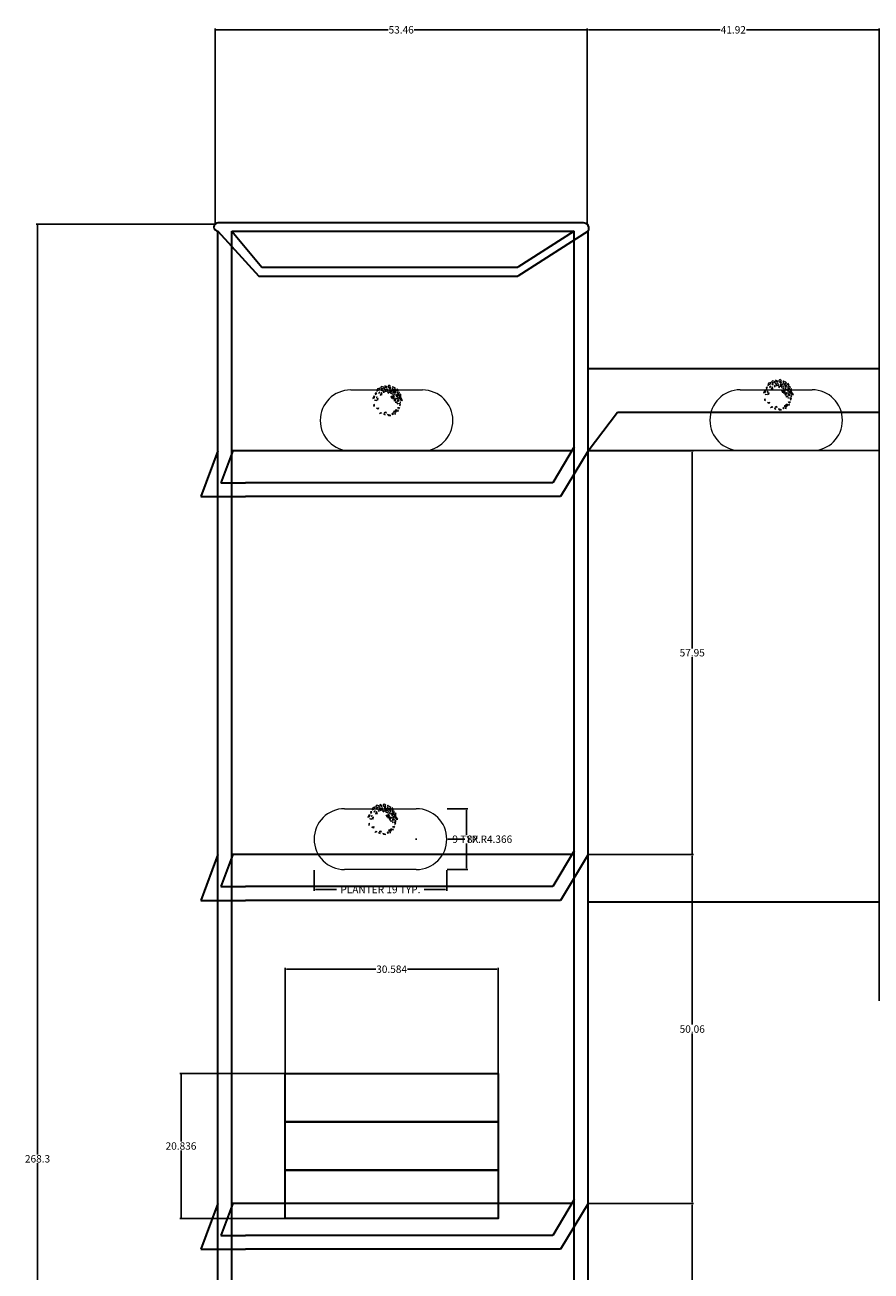
# Model space of a CAD drawing. Units: inches. Extents: x 35 to 365, y 67 to 380.
# Tile 2 of 5: x 35 to 156, y 201 to 380. Entities that reach past the tile are written whole.
import ezdxf

# ---------------------------------------------------------------- set-up
doc = ezdxf.new("R2010")
doc.units = ezdxf.units.IN
doc.header["$MEASUREMENT"] = 0
for name, color, linetype, lineweight in [('A-ANNO-DIMS', 2, 'Continuous', 18), ('A-FURN', 7, 'Continuous', 35), ('A-FURN-PLNT', 3, 'Continuous', 13)]:
    doc.layers.add(name, color=color, linetype=linetype, lineweight=lineweight)
doc.styles.get("Standard").update_dxf_attribs({"font": 'arial.ttf'})
doc.dimstyles.get("Standard").update_dxf_attribs({"dimtxt": 1.0625, "dimasz": 0.18, "dimexe": 0.18, "dimexo": 0.0625, "dimgap": 0.09, "dimtad": 0, "dimtih": 1, "dimtoh": 1, "dimdec": 4, "dimzin": 0, "dimdsep": 46, "dimlunit": 4, "dimtxsty": 'Standard', "dimcen": 0.09, "dimadec": 0, "dimazin": 0, "dimtfac": 1, "dimtdec": 4, "dimtofl": 0, "dimtmove": 0, "dimatfit": 3, "dimfxl": 1, "dimtolj": 1, "dimtzin": 0, "dimarcsym": 0})

# ---------------------------------------------------------------- blocks, each defined once
blk = doc.blocks.new('*U2')
for points in [[(-5.78, 9.75), (-7.54, 9.23), (-8.01, 7.5), (-6.26, 8.45)], [(-4.43, 11.05), (-5.18, 10.36), (-3.96, 9.49), (-2.07, 10.36)], [(-2, 11.66), (-1.6, 10.62), (-0.52, 10.1), (-0.18, 10.62), (-0.79, 10.96)], [(1.24, 12), (0.56, 11.31), (0.76, 10.01), (2.52, 11.05)], [(2.59, 9.93), (1.84, 9.75), (1.64, 9.23), (2.32, 9.41)], [(4.14, 11.14), (3.6, 10.01), (4, 9.23), (5.22, 8.71), (6.3, 9.41), (5.08, 10.19), (4.61, 10.01)], [(-11.32, 1.79), (-9.83, 2.31), (-9.63, 3.44), (-10.44, 3.52)], [(-8.21, 0.41), (-9.43, 0.32), (-9.83, 0.84)], [(-8.14, 6.03), (-9.36, 5.95), (-9.02, 4.73)], [(-8.21, 3.09), (-8.48, 2.31), (-7.87, 2.57)], [(-7, 1.79), (-7.94, 1.53), (-7.47, 0.49)], [(-5.78, 6.81), (-6.66, 6.21), (-6.52, 5.69)], [(-4.57, 6.38), (-5.45, 4.47), (-3.89, 4.82)], [(-4.84, 8.63), (-3.83, 7.85), (-4.03, 8.97)], [(-2.88, 7.5), (-3.15, 6.64), (-2.27, 6.72)], [(-1.94, 9.49), (-2.48, 8.97), (-2.27, 8.54), (-1.8, 9.06)], [(0.02, 9.06), (-1.33, 8.54), (-1.73, 7.16), (0.29, 7.76)], [(0.76, 7.16), (0.09, 6.46), (1.1, 5.95)], [(1.37, 8.54), (3.13, 8.8), (3.8, 7.85), (1.91, 7.76)], [(1.71, 6.29), (1.71, 7.07), (2.65, 7.5), (2.11, 6.9)], [(2.52, 6.81), (2.52, 5.86), (4.41, 5.17), (4.61, 6.72)], [(3.53, 1.88), (2.86, 3.52), (3.8, 3.52)], [(4.41, 4.56), (4.27, 3.7), (5.49, 3.26)], [(4.27, 2.74), (5.29, 2.66), (4.41, 1.27)], [(4.61, 8.28), (4.54, 7.76), (4.95, 7.59), (4.95, 8.28)], [(5.83, 1.53), (5.02, 0.41), (5.49, -0.02), (6.5, 0.41)], [(5.49, 5.51), (5.42, 4.82), (6.16, 5.08)], [(6.43, 7.94), (5.49, 7.68), (5.56, 6.21), (6.5, 6.64)], [(7.51, 1.71), (6.91, 1.27), (6.23, 2.14)], [(8.12, 4.99), (7.11, 4.65), (6.5, 4.13), (7.38, 3.09), (8.12, 3.52), (7.65, 3.87)], [(7.45, 9.32), (7.11, 7.94), (8.52, 7.94)], [(7.85, 6.81), (7.18, 6.21), (9, 5.51), (9.33, 6.38)], [(8.12, 0.75), (7.51, 0.15), (8.93, -0.28), (9.13, 0.49)], [(8.19, 2.57), (7.92, 2.05), (8.66, 1.53)], [(8.73, 4.73), (8.19, 4.56), (8.39, 3.87), (8.59, 4.04)], [(10.28, 5.17), (9.2, 4.04), (9, 2.31), (10.48, 0.49), (11.76, 0.41), (10.35, 2.48), (9.33, 2.4), (10.28, 2.83)], [(-10.03, -2.71), (-10.64, -3.31), (-10.44, -4.44), (-9.9, -3.49)], [(-8.28, -5.73), (-6.79, -5.3), (-7, -6.51)], [(-4.84, -8.85), (-4.43, -9.45), (-5.99, -9.8)], [(-2.34, -9.2), (-1.26, -8.5), (-0.99, -9.54)], [(4.07, -9.45), (3.53, -9.97), (4.07, -10.58), (4.61, -9.89)], [(5.29, -7.98), (4.61, -8.16), (5.02, -8.94)], [(6.03, -9.45), (5.42, -9.97), (6.16, -10.15)], [(6.1, -8.94), (6.16, -7.21), (6.91, -6.69), (7.24, -7.38)], [(7.78, -0.8), (6.43, -1.5), (6.43, -0.72)], [(8.32, -1.75), (7.98, -2.53), (7.58, -2.1)], [(8.05, -8.07), (8.59, -7.12), (7.92, -7.55)], [(9.33, -5.13), (8.46, -6.25), (7.98, -5.22)], [(9.33, -1.75), (9.54, -3.74), (10.14, -2.53)], [(10.08, -0.63), (9.74, -1.32), (10.48, -0.89)], [(-2.54, -10.06), (-3.02, -10.23), (-1.8, -10.67)], [(0.22, -10.58), (0.83, -11.27), (2.59, -11.36)]]:
    blk.add_lwpolyline(points, close=True)
blk = doc.blocks.new('SHELF-GLASS')
for p, q in [((2.48, 6.58), (0, 0)), ((4.62, 6.58), (2.89, 2)), ((53.29, 6.58), (4.62, 6.58)), ((53.63, 7.13), (50.54, 2)), ((55.63, 6.58), (51.68, 0)), ((2.89, 2), (6.44, 2)), ((50.54, 2), (6.44, 2)), ((0, 0), (6.44, 0)), ((51.68, 0), (6.44, 0))]:
    blk.add_line(p, q)
blk = doc.blocks.new('PLANTER')
for points in [[(4.37, 8.73), (14.67, 8.73)], [(14.67, 0), (4.37, 0)]]:
    blk.add_lwpolyline(points)
for centre, start, end in [((4.37, 4.37), 90, 270), ((14.67, 4.37), 270, 90)]:
    blk.add_arc(centre, 4.37, start, end)
blk = doc.blocks.new('*D5')
at = {"layer": 'A-ANNO-DIMS', "color": 0, "lineweight": -2, "transparency": 16777216}
for p, q in [((76.04, 258.65), (76.04, 255.68)), ((95.08, 258.65), (95.08, 255.68)), ((76.22, 255.86), (79.28, 255.86)), ((94.9, 255.86), (91.84, 255.86))]:
    blk.add_line(p, q, dxfattribs=at)
at = {"layer": 'A-ANNO-DIMS', "color": 0, "transparency": 16777216}
for points in [[(76.22, 255.89), (76.22, 255.83), (76.04, 255.86)], [(94.9, 255.89), (94.9, 255.83), (95.08, 255.86)]]:
    blk.add_solid(points, dxfattribs=at)
at = {"layer": 'Defpoints', "color": 0, "transparency": 16777216}
for p in [(76.04, 258.72), (95.08, 258.72), (95.08, 255.86)]:
    blk.add_point(p, dxfattribs=at)
at = {"layer": 'A-ANNO-DIMS', "color": 0, "transparency": 16777216, "insert": (85.56, 255.86), "char_height": 1.0625, "attachment_point": 5}
blk.add_mtext('\\A1;PLANTER 19 TYP.', dxfattribs=at)
blk = doc.blocks.new('*D6')
at = {"layer": 'A-ANNO-DIMS', "color": 0, "lineweight": -2, "transparency": 16777216}
for p, q in [((95.14, 267.45), (98.11, 267.45)), ((97.93, 267.27), (97.93, 263.72)), ((97.93, 258.9), (97.93, 262.45)), ((95.14, 258.72), (98.11, 258.72))]:
    blk.add_line(p, q, dxfattribs=at)
at = {"layer": 'A-ANNO-DIMS', "color": 0, "transparency": 16777216}
for points in [[(97.9, 267.27), (97.96, 267.27), (97.93, 267.45)], [(97.9, 258.9), (97.96, 258.9), (97.93, 258.72)]]:
    blk.add_solid(points, dxfattribs=at)
at = {"layer": 'Defpoints', "color": 0, "transparency": 16777216}
for p in [(95.08, 267.45), (97.93, 267.45), (95.08, 258.72)]:
    blk.add_point(p, dxfattribs=at)
at = {"layer": 'A-ANNO-DIMS', "color": 0, "transparency": 16777216, "insert": (97.93, 263.08), "char_height": 1.062, "attachment_point": 5}
blk.add_mtext('\\A1;9 TYP.', dxfattribs=at)
blk = doc.blocks.new('*D10')
at = {"layer": 'A-ANNO-DIMS', "color": 0, "lineweight": -2, "transparency": 16777216}
for p, q in [((61.75, 351.36), (36.15, 351.36)), ((36.33, 351.18), (36.33, 217.84)), ((36.33, 83.23), (36.33, 216.57)), ((61.26, 83.05), (36.15, 83.05))]:
    blk.add_line(p, q, dxfattribs=at)
at = {"layer": 'A-ANNO-DIMS', "color": 0, "transparency": 16777216}
for points in [[(36.3, 351.18), (36.36, 351.18), (36.33, 351.36)], [(36.3, 83.23), (36.36, 83.23), (36.33, 83.05)]]:
    blk.add_solid(points, dxfattribs=at)
at = {"layer": 'Defpoints', "color": 0, "transparency": 16777216}
for p in [(36.33, 351.36), (61.82, 351.36), (61.32, 83.05)]:
    blk.add_point(p, dxfattribs=at)
at = {"layer": 'A-ANNO-DIMS', "color": 0, "transparency": 16777216, "insert": (36.33, 217.21), "char_height": 1.062, "attachment_point": 5}
blk.add_mtext('\\A1;268.3', dxfattribs=at)
blk = doc.blocks.new('*D11')
at = {"layer": 'A-ANNO-DIMS', "color": 0, "lineweight": -2, "transparency": 16777216}
for p, q in [((61.82, 351.42), (61.82, 379.42)), ((62, 379.24), (86.66, 379.24)), ((115.09, 379.24), (90.43, 379.24)), ((115.27, 351.36), (115.27, 379.42))]:
    blk.add_line(p, q, dxfattribs=at)
at = {"layer": 'A-ANNO-DIMS', "color": 0, "transparency": 16777216}
for points in [[(62, 379.27), (62, 379.21), (61.82, 379.24)], [(115.09, 379.27), (115.09, 379.21), (115.27, 379.24)]]:
    blk.add_solid(points, dxfattribs=at)
at = {"layer": 'Defpoints', "color": 0, "transparency": 16777216}
for p in [(115.27, 379.24), (61.82, 351.36), (115.27, 351.3)]:
    blk.add_point(p, dxfattribs=at)
at = {"layer": 'A-ANNO-DIMS', "color": 0, "transparency": 16777216, "insert": (88.54, 379.24), "char_height": 1.062, "attachment_point": 5}
blk.add_mtext('\\A1;53.46', dxfattribs=at)
blk = doc.blocks.new('*D12')
at = {"layer": 'A-ANNO-DIMS', "color": 0, "lineweight": -2, "transparency": 16777216}
for p, q in [((115.27, 351.36), (115.27, 379.42)), ((115.45, 379.24), (134.33, 379.24)), ((157.01, 379.24), (138.13, 379.24)), ((157.19, 239.87), (157.19, 379.42))]:
    blk.add_line(p, q, dxfattribs=at)
at = {"layer": 'A-ANNO-DIMS', "color": 0, "transparency": 16777216}
for points in [[(115.45, 379.27), (115.45, 379.21), (115.27, 379.24)], [(157.01, 379.27), (157.01, 379.21), (157.19, 379.24)]]:
    blk.add_solid(points, dxfattribs=at)
at = {"layer": 'Defpoints', "color": 0, "transparency": 16777216}
for p in [(157.19, 379.24), (115.27, 351.3), (157.19, 239.81)]:
    blk.add_point(p, dxfattribs=at)
at = {"layer": 'A-ANNO-DIMS', "color": 0, "transparency": 16777216, "insert": (136.23, 379.24), "char_height": 1.062, "attachment_point": 5}
blk.add_mtext('\\A1;41.92', dxfattribs=at)
blk = doc.blocks.new('*D32')
at = {"layer": 'A-ANNO-DIMS', "color": 0, "lineweight": -2, "transparency": 16777216}
for p, q in [((71.88, 229.53), (71.88, 244.6)), ((72.06, 244.42), (84.88, 244.42)), ((102.29, 244.42), (89.47, 244.42)), ((102.47, 229.53), (102.47, 244.6))]:
    blk.add_line(p, q, dxfattribs=at)
at = {"layer": 'A-ANNO-DIMS', "color": 0, "transparency": 16777216}
for points in [[(72.06, 244.45), (72.06, 244.39), (71.88, 244.42)], [(102.29, 244.45), (102.29, 244.39), (102.47, 244.42)]]:
    blk.add_solid(points, dxfattribs=at)
at = {"layer": 'Defpoints', "color": 0, "transparency": 16777216}
for p in [(102.47, 244.42), (71.88, 229.47), (102.47, 229.47)]:
    blk.add_point(p, dxfattribs=at)
at = {"layer": 'A-ANNO-DIMS', "color": 0, "transparency": 16777216, "insert": (87.17, 244.42), "char_height": 1.062, "attachment_point": 5}
blk.add_mtext('\\A1;30.584', dxfattribs=at)
blk = doc.blocks.new('*D33')
at = {"layer": 'A-ANNO-DIMS', "color": 0, "lineweight": -2, "transparency": 16777216}
for p, q in [((71.82, 229.47), (56.75, 229.47)), ((56.93, 229.29), (56.93, 219.68)), ((56.93, 208.81), (56.93, 218.41)), ((71.82, 208.63), (56.75, 208.63))]:
    blk.add_line(p, q, dxfattribs=at)
at = {"layer": 'A-ANNO-DIMS', "color": 0, "transparency": 16777216}
for points in [[(56.9, 229.29), (56.96, 229.29), (56.93, 229.47)], [(56.9, 208.81), (56.96, 208.81), (56.93, 208.63)]]:
    blk.add_solid(points, dxfattribs=at)
at = {"layer": 'Defpoints', "color": 0, "transparency": 16777216}
for p in [(56.93, 229.47), (71.88, 229.47), (71.88, 208.63)]:
    blk.add_point(p, dxfattribs=at)
at = {"layer": 'A-ANNO-DIMS', "color": 0, "transparency": 16777216, "insert": (56.93, 219.05), "char_height": 1.062, "attachment_point": 5}
blk.add_mtext('\\A1;20.836', dxfattribs=at)
blk = doc.blocks.new('*D35')
at = {"layer": 'A-ANNO-DIMS', "color": 0, "lineweight": -2, "transparency": 16777216}
for p, q in [((115.45, 210.8), (130.51, 210.8)), ((130.33, 210.62), (130.33, 186.09)), ((130.33, 160.29), (130.33, 184.82)), ((115.45, 160.11), (130.51, 160.11))]:
    blk.add_line(p, q, dxfattribs=at)
at = {"layer": 'A-ANNO-DIMS', "color": 0, "transparency": 16777216}
for points in [[(130.3, 210.62), (130.36, 210.62), (130.33, 210.8)], [(130.3, 160.29), (130.36, 160.29), (130.33, 160.11)]]:
    blk.add_solid(points, dxfattribs=at)
at = {"layer": 'Defpoints', "color": 0, "transparency": 16777216}
for p in [(115.38, 210.8), (115.38, 160.11), (130.33, 160.11)]:
    blk.add_point(p, dxfattribs=at)
at = {"layer": 'A-ANNO-DIMS', "color": 0, "transparency": 16777216, "insert": (130.33, 185.46), "char_height": 1.062, "attachment_point": 5}
blk.add_mtext('\\A1;50.69', dxfattribs=at)
blk = doc.blocks.new('*D36')
at = {"layer": 'A-ANNO-DIMS', "color": 0, "lineweight": -2, "transparency": 16777216}
for p, q in [((115.45, 260.87), (130.51, 260.87)), ((130.33, 260.69), (130.33, 236.47)), ((130.33, 210.98), (130.33, 235.2)), ((115.45, 210.8), (130.51, 210.8))]:
    blk.add_line(p, q, dxfattribs=at)
at = {"layer": 'A-ANNO-DIMS', "color": 0, "transparency": 16777216}
for points in [[(130.3, 260.69), (130.36, 260.69), (130.33, 260.87)], [(130.3, 210.98), (130.36, 210.98), (130.33, 210.8)]]:
    blk.add_solid(points, dxfattribs=at)
at = {"layer": 'Defpoints', "color": 0, "transparency": 16777216}
for p in [(115.38, 260.87), (115.38, 210.8), (130.33, 210.8)]:
    blk.add_point(p, dxfattribs=at)
at = {"layer": 'A-ANNO-DIMS', "color": 0, "transparency": 16777216, "insert": (130.33, 235.83), "char_height": 1.062, "attachment_point": 5}
blk.add_mtext('\\A1;50.06', dxfattribs=at)
blk = doc.blocks.new('*D37')
at = {"layer": 'A-ANNO-DIMS', "color": 0, "lineweight": -2, "transparency": 16777216}
for p, q in [((115.45, 318.82), (130.51, 318.82)), ((130.33, 318.64), (130.33, 290.47)), ((130.33, 261.05), (130.33, 289.21)), ((115.45, 260.87), (130.51, 260.87))]:
    blk.add_line(p, q, dxfattribs=at)
at = {"layer": 'A-ANNO-DIMS', "color": 0, "transparency": 16777216}
for points in [[(130.3, 318.64), (130.36, 318.64), (130.33, 318.82)], [(130.3, 261.05), (130.36, 261.05), (130.33, 260.87)]]:
    blk.add_solid(points, dxfattribs=at)
at = {"layer": 'Defpoints', "color": 0, "transparency": 16777216}
for p in [(115.38, 318.82), (115.38, 260.87), (130.33, 260.87)]:
    blk.add_point(p, dxfattribs=at)
at = {"layer": 'A-ANNO-DIMS', "color": 0, "transparency": 16777216, "insert": (130.33, 289.84), "char_height": 1.062, "attachment_point": 5}
blk.add_mtext('\\A1;57.95', dxfattribs=at)
blk = doc.blocks.new('*D38')
at = {"layer": 'A-ANNO-DIMS', "color": 0, "lineweight": -2, "transparency": 16777216}
for p, q in [((90.62, 263.08), (90.8, 263.08)), ((90.71, 262.99), (90.71, 263.17)), ((97.7, 263.08), (95.26, 263.08))]:
    blk.add_line(p, q, dxfattribs=at)
at = {"layer": 'A-ANNO-DIMS', "color": 0, "transparency": 16777216}
blk.add_solid([(95.26, 263.11), (95.26, 263.05), (95.08, 263.08)], dxfattribs=at)
at = {"layer": 'Defpoints', "color": 0, "transparency": 16777216}
for p in [(90.71, 263.08), (95.08, 263.08)]:
    blk.add_point(p, dxfattribs=at)
at = {"layer": 'A-ANNO-DIMS', "color": 0, "transparency": 16777216, "insert": (101.23, 263.08), "char_height": 1.0625, "attachment_point": 5}
blk.add_mtext('\\A1;8X R4.366', dxfattribs=at)

msp = doc.modelspace()

# ---------------------------------------------------------------- linework, layer by layer
at = {"layer": 'A-FURN'}
for p, q in [((114.7118, 351.5361), (62.2395, 351.5361)), ((62.2395, 122.4805), (62.2395, 350.3365)), ((62.2395, 350.3365), (68.1196, 343.8794)), ((64.2395, 122.4805), (64.2395, 350.3365)), ((64.2395, 350.3365), (68.5378, 345.1789)), ((64.2395, 350.3365), (113.383, 350.3365)), ((115.383, 350.3365), (105.2791, 343.8794)), ((113.383, 350.3365), (105.3126, 345.1789)), ((113.383, 123.0351), (113.383, 350.3365)), ((115.383, 122.4805), (115.383, 350.3365)), ((68.5378, 345.1789), (105.3126, 345.1789)), ((68.1196, 343.8794), (105.2791, 343.8794)), ((115.383, 330.6506), (323.6655, 330.6506)), ((115.383, 318.8192), (119.5786, 324.3612)), ((119.5786, 324.3612), (317.6655, 324.3612)), ((62.2395, 318.8192), (59.756, 312.2417)), ((64.3773, 318.8192), (62.649, 314.2417)), ((113.0498, 318.8192), (64.3773, 318.8192)), ((113.383, 319.3738), (110.2998, 314.2417)), ((115.383, 318.8192), (111.4314, 312.2417)), ((323.6655, 319.0524), (115.383, 318.8192)), ((62.649, 314.2417), (66.1912, 314.2417)), ((110.2998, 314.2417), (66.1912, 314.2417)), ((59.756, 312.2417), (66.1912, 312.2417)), ((111.4314, 312.2417), (66.1912, 312.2417))]:
    msp.add_line(p, q, dxfattribs=at)
for points in [[(115.383, 254.0695), (323.6655, 254.0695), (323.6655, 151.0198), (115.383, 151.0198)], [(71.8824, 229.4659), (102.4669, 229.4659), (102.4669, 222.5205), (71.8824, 222.5205)], [(71.8824, 222.5205), (102.4669, 222.5205), (102.4669, 215.575), (71.8824, 215.575)], [(71.8824, 215.575), (102.4669, 215.575), (102.4669, 208.6296), (71.8824, 208.6296)]]:
    msp.add_lwpolyline(points, close=True, dxfattribs=at)
for centre, radius, start, end in [((62.2395, 350.9363), 0.5998, 90, 270), ((114.7118, 350.7485), 0.7876, 328.460951, 90)]:
    msp.add_arc(centre, radius, start, end, dxfattribs=at)

# ---------------------------------------------------------------- block references
for p in [(59.756, 254.2875), (59.756, 204.2249)]:
    msp.add_blockref('SHELF-GLASS', p, dxfattribs=at)
at = {"layer": 'A-FURN-PLNT', "rotation": 180}
for p in [(95.9607, 327.5521), (151.9017, 327.5823)]:
    msp.add_blockref('PLANTER', p, dxfattribs=at)
at = {"layer": 'A-FURN-PLNT', "xscale": 0.1863493069736422, "yscale": 0.1863493069736422, "zscale": 0.1863493069736422}
for p in [(86.5589, 325.9869), (142.6788, 326.8071), (85.8626, 265.8851)]:
    msp.add_blockref('*U2', p, dxfattribs=at)
at = {"layer": 'A-FURN-PLNT'}
msp.add_blockref('PLANTER', (76.043, 258.717), dxfattribs=at)

# ---------------------------------------------------------------- dimensions: what is measured, and where the dimension line sits
at = {"layer": 'A-ANNO-DIMS'}
for base, p1, p2, override, picture, middle in [((115.273, 379.2444), (61.8154, 351.3604), (115.273, 351.3011), {"dimdec": 2, "dimlfac": 1, "dimrnd": 0, "dimzin": 0, "dimdsep": 46, "dimlunit": 2}, '*D11', (88.5442, 379.2444)), ((157.1904, 379.2444), (115.273, 351.3011), (157.1904, 239.8076), {"dimdec": 2, "dimlfac": 1, "dimrnd": 0, "dimzin": 0, "dimdsep": 46, "dimlunit": 2}, '*D12', (136.2317, 379.2444)), ((102.46692, 244.41591), (71.88243, 229.46591), (102.46692, 229.46591), {"dimdec": 3, "dimlfac": 1, "dimrnd": 0, "dimzin": 0, "dimdsep": 46, "dimlunit": 2}, '*D32', (87.17468, 244.41591))]:
    dim = msp.add_linear_dim(base=base, p1=p1, p2=p2, dimstyle='Standard', override=override, dxfattribs=at)
    dim.commit()
    dim.dimension.update_dxf_attribs({"geometry": picture, "text_midpoint": middle})
for base, p1, p2, angle, override, picture, middle in [((36.3297, 351.3604), (61.3227, 83.0529), (61.8154, 351.3604), 90, {"dimdec": 1, "dimlfac": 1, "dimrnd": 0, "dimzin": 0, "dimdsep": 46, "dimlunit": 2}, '*D10', (36.3297, 217.2067)), ((130.333, 260.8654), (115.383, 318.8192), (115.383, 260.8654), 270, {"dimdec": 2, "dimlfac": 1, "dimrnd": 0, "dimzin": 0, "dimdsep": 46, "dimlunit": 2}, '*D37', (130.333, 289.8423)), ((130.333, 210.8028), (115.383, 260.8654), (115.383, 210.8028), 270, {"dimdec": 2, "dimlfac": 1, "dimrnd": 0, "dimzin": 0, "dimdsep": 46, "dimlunit": 2}, '*D36', (130.333, 235.8341)), ((56.9324, 229.4659), (71.8824, 208.6296), (71.8824, 229.4659), 90, {"dimdec": 3, "dimlfac": 1, "dimrnd": 0, "dimzin": 0, "dimdsep": 46, "dimlunit": 2}, '*D33', (56.9324, 219.0477)), ((130.333, 160.1089), (115.383, 210.8028), (115.383, 160.1089), 270, {"dimdec": 2, "dimlfac": 1, "dimrnd": 0, "dimzin": 0, "dimdsep": 46, "dimlunit": 2}, '*D35', (130.333, 185.4559))]:
    dim = msp.add_linear_dim(base=base, p1=p1, p2=p2, angle=angle, dimstyle='Standard', override=override, dxfattribs=at)
    dim.commit()
    dim.dimension.update_dxf_attribs({"geometry": picture, "text_midpoint": middle})
dim = msp.add_linear_dim(base=(97.9308, 267.4499), p1=(95.0759, 258.7174), p2=(95.0759, 267.4499), angle=90, text='<> TYP.', dimstyle='Standard', override={"dimdec": 0, "dimrnd": 0, "dimzin": 0, "dimlunit": 2}, dxfattribs=at)
dim.commit()
dim.dimension.update_dxf_attribs({"geometry": '*D6', "text_midpoint": (97.9308, 263.0836)})
dim = msp.add_radius_dim(center=(90.7096, 263.0836), mpoint=(95.0759, 263.084), text='8X <>', dimstyle='Standard', override={"dimdec": 3, "dimlfac": 1, "dimrnd": 0, "dimzin": 0, "dimdsep": 46, "dimlunit": 2}, dxfattribs=at)
dim.commit()
dim.dimension.update_dxf_attribs({"geometry": '*D38', "text_midpoint": (97.6956, 263.0842), "dimtype": 164})
dim = msp.add_linear_dim(base=(95.0759, 255.8624), p1=(76.0432, 258.7174), p2=(95.0759, 258.7174), text='PLANTER <> TYP.', dimstyle='Standard', override={"dimdec": 0, "dimrnd": 0, "dimzin": 0, "dimlunit": 2}, dxfattribs=at)
dim.commit()
dim.dimension.update_dxf_attribs({"geometry": '*D5', "text_midpoint": (85.5595, 255.8624)})

doc.saveas('drawing.dxf')
